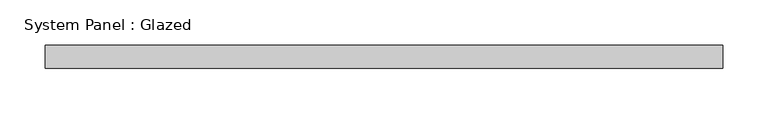
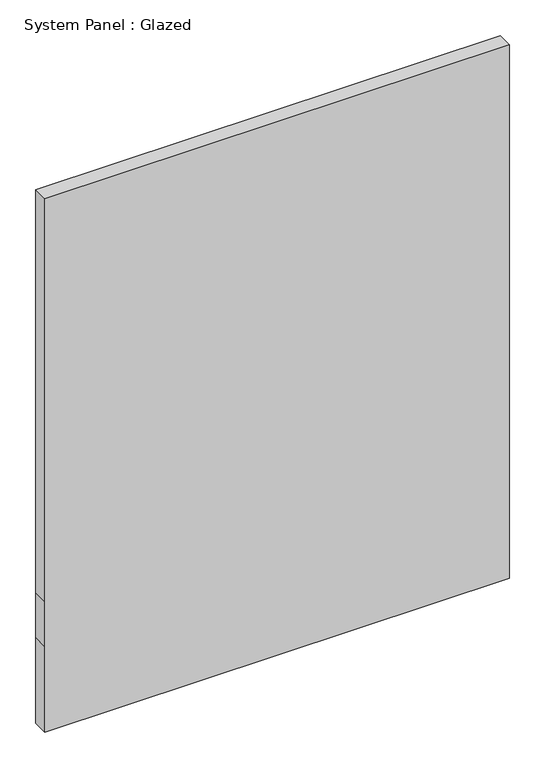
"""IFC4 building model written with IfcOpenShell, lengths in millimetres: plate geometry, System Panel : Glazed."""

from ifc_helpers import new_model, si_unit, frame, origin, place, context, project, spatial, polyline, outline, extrude, source, transform, mapped, element, save


def system_panel_glazed_3f655f72(model_context):
    return source(origin(), model_context, "Body", "SweptSolid", [
        extrude(outline(polyline([(0.0, -374.65), (0.0, 374.65), (146.05, 374.65), (222.25, 374.65), (909.366916, 374.65), (909.366916, -374.65), (222.25, -374.65), (146.05, -374.65), (0.0, -374.65)])), frame((0.0, 19.05, 0.0), z_axis=(0.0, 1.0, 0.0), x_axis=(0.0, 0.0, 1.0)), (0.0, 0.0, 1.0), 25.4),
    ])


if __name__ == "__main__":
    model = new_model("IFC4")
    model_context = context("Model", 3, world=origin())
    ifc_project = project(units=[si_unit("LENGTHUNIT", "METRE", prefix="MILLI")], contexts=[model_context])
    site = spatial("IfcSite", under=ifc_project)
    building = spatial("IfcBuilding", under=site)
    placement = place(None, origin())
    system_panel_glazed_shape = system_panel_glazed_3f655f72(model_context)
    element("IfcPlate", 1, ObjectType="System Panel : Glazed", at=placement, inside=building, context=model_context, shape_type="MappedRepresentation", body=[
        mapped(system_panel_glazed_shape, transform((0.0, 0.0, 0.0), x_axis=(1.0, 0.0, 0.0), y_axis=(0.0, 1.0, 0.0), z_axis=(0.0, 0.0, 1.0))),
    ])
    save(model, "model.ifc")

# Revit data of these elements
# Type "System Panel : Glazed"
#   Construction Type Id = "GSP4R"
#   Analytic Construction = "1/8 in Pilkington single glazing"
#   Visual Light Transmittance = 0.9
#   Solar Heat Gain Coefficient = 0.86
#   Heat Transfer Coefficient (U) = 1.18115 BTU/(h·ft²·°F)
#   Define Thermal Properties by = 1
# Element 1 (IfcPlate, "System Panel : Glazed")
#   Materials on its faces: "Glass"
# Materials
#   "Glass": class "Glass", colour RGB 0 128 192, transparency 0.75, Description = "Soda Lime Glass", Cost = 0
